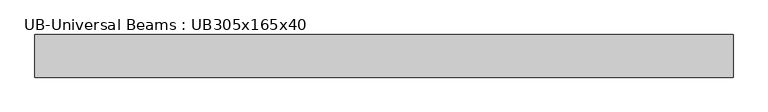
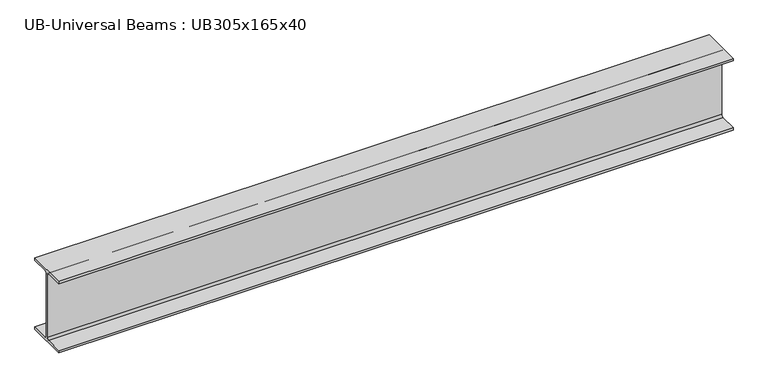
"""IFC4 building model written with IfcOpenShell, lengths in millimetres: beam geometry, UB-Universal Beams : UB305x165x40."""

from ifc_helpers import new_model, si_unit, point, frame, frame_2d, origin, place, context, project, spatial, polyline, circle_curve, trimmed, segment, composite_curve, outline, extrude, source, transform, mapped, element, save


def ub_universal_beams_ub305x165x40_8fd3c0bc(model_context):
    return source(origin(), model_context, "Body", "SweptSolid", [
        extrude(outline(composite_curve([segment(polyline([(82.5, -141.5), (82.5, -151.7), (-82.5, -151.7), (-82.5, -141.5), (-11.9, -141.5)]), True, "CONTINUOUS"), segment(trimmed(circle_curve(frame_2d((-11.9, -132.6)), 8.9), [point((-11.9, -141.5))], [point((-3.0, -132.6))], True, "CARTESIAN"), True, "CONTINUOUS"), segment(polyline([(-3.0, -132.6), (-3.0, 132.6)]), True, "CONTINUOUS"), segment(trimmed(circle_curve(frame_2d((-11.9, 132.6)), 8.9), [point((-3.0, 132.6))], [point((-11.9, 141.5))], True, "CARTESIAN"), True, "CONTINUOUS"), segment(polyline([(-11.9, 141.5), (-82.5, 141.5), (-82.5, 151.7), (82.5, 151.7), (82.5, 141.5), (11.9, 141.5)]), True, "CONTINUOUS"), segment(trimmed(circle_curve(frame_2d((11.9, 132.6)), 8.9), [point((11.9, 141.5))], [point((3.0, 132.6))], True, "CARTESIAN"), True, "CONTINUOUS"), segment(polyline([(3.0, 132.6), (3.0, -132.6)]), True, "CONTINUOUS"), segment(trimmed(circle_curve(frame_2d((11.9, -132.6)), 8.9), [point((3.0, -132.6))], [point((11.9, -141.5))], True, "CARTESIAN"), True, "CONTINUOUS"), segment(polyline([(11.9, -141.5), (82.5, -141.5)]), True, "CONTINUOUS")], self_intersect=False)), frame((-1302.3, 0.0, 0.0), z_axis=(1.0, 0.0, 0.0), x_axis=(0.0, 1.0, 0.0)), (0.0, 0.0, 1.0), 2703.9),
    ])


if __name__ == "__main__":
    model = new_model("IFC4")
    model_context = context("Model", 3, world=origin())
    ifc_project = project(units=[si_unit("LENGTHUNIT", "METRE", prefix="MILLI")], contexts=[model_context])
    site = spatial("IfcSite", under=ifc_project)
    building = spatial("IfcBuilding", under=site)
    placement = place(None, origin())
    ub_universal_beams_ub305x165x40_shape = ub_universal_beams_ub305x165x40_8fd3c0bc(model_context)
    element("IfcBeam", 1, ObjectType="UB-Universal Beams : UB305x165x40", at=placement, inside=building, context=model_context, shape_type="MappedRepresentation", body=[
        mapped(ub_universal_beams_ub305x165x40_shape, transform((0.0, 0.0, 0.0), x_axis=(1.0, 0.0, 0.0), y_axis=(0.0, 1.0, 0.0), z_axis=(0.0, 0.0, 1.0))),
    ])
    save(model, "model.ifc")

# Revit data of these elements
# Type "UB-Universal Beams : UB305x165x40"
#   Section Name Key = "UB305X165X40"
#   Width = 16.5 cm
#   Web Thickness = 0.6 cm
#   Web Fillet = 0.89 cm
#   Warping Constant = 164000.0 cm⁶
#   Torsional Moment of Inertia = 14.70 cm⁴
#   Section Area = 51.3 cm²
#   Plastic Modulus weak axis = 142.0 cm³
#   Plastic Modulus strong axis = 623.0 cm³
#   Nominal Weight = 40.2999 kgf/m
#   Moment of Inertia weak axis = 764.00 cm⁴
#   Moment of Inertia strong axis = 8503.00 cm⁴
#   Height = 30.34 cm
#   Flange Thickness = 1.02 cm
#   Elastic Modulus weak axis = 92.6 cm³
#   Elastic Modulus strong axis = 560.0 cm³
#   Centroid Vertical = 15.17 cm
#   Centroid Horizontal = 8.25 cm
#   Bolt Spacing = 9.0 cm
#   Length [instance default] = 1500 mm
#   Structural Material [instance default] = Metal - Steel 43-275
#   Type Comments = ""
#   Assembly Code = ""
# Element 1 (IfcBeam, "UB-Universal Beams : UB305x165x40")
#   Materials on its faces: "Metal - Steel 43-275"
# Materials
#   "Metal - Steel 43-275": class "Metal", colour RGB 247 247 247, transparency 0, Cost = 0
